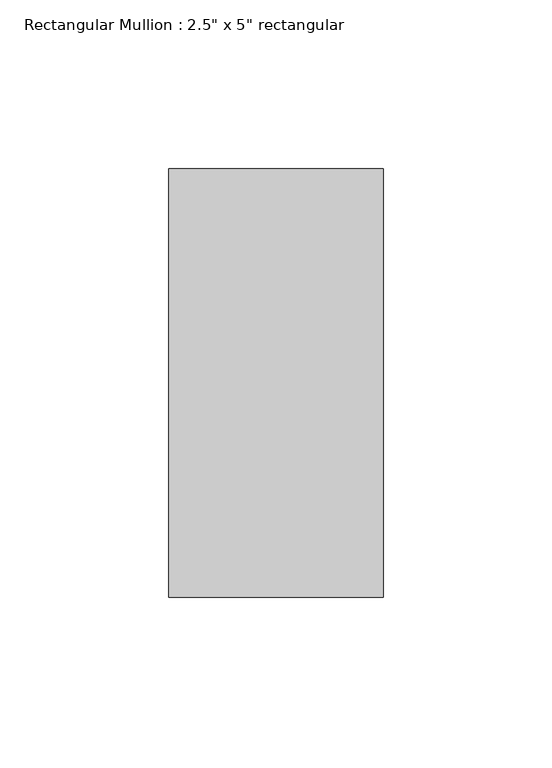
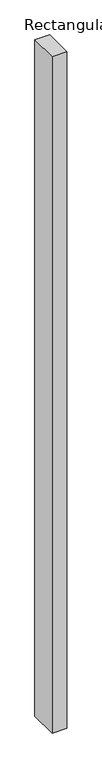
"""IFC4 building model written with IfcOpenShell, lengths in millimetres: member geometry."""

from ifc_helpers import new_model, si_unit, frame, origin, place, context, project, spatial, polyline, outline, extrude, source, transform, mapped, element, save


def member_3f395ae9(model_context):
    return source(origin(), model_context, "Body", "SweptSolid", [
        extrude(outline(polyline([(0.0, 63.5), (0.0, -63.5), (-63.5, -63.5), (-63.5, 63.5), (0.0, 63.5)])), frame((0.0, 0.0, -3048.0), z_axis=(0.0, 0.0, 1.0), x_axis=(1.0, 0.0, 0.0)), (0.0, 0.0, 1.0), 3048.0),
    ])


if __name__ == "__main__":
    model = new_model("IFC4")
    model_context = context("Model", 3, world=origin())
    ifc_project = project(units=[si_unit("LENGTHUNIT", "METRE", prefix="MILLI")], contexts=[model_context])
    site = spatial("IfcSite", under=ifc_project)
    building = spatial("IfcBuilding", under=site)
    placement = place(None, origin())
    member_shape = member_3f395ae9(model_context)
    element("IfcMember", 1, ObjectType="Rectangular Mullion : 2.5\" x 5\" rectangular", at=placement, inside=building, context=model_context, shape_type="MappedRepresentation", body=[
        mapped(member_shape, transform((0.0, 0.0, 0.0), x_axis=(1.0, 0.0, 0.0), y_axis=(0.0, 1.0, 0.0), z_axis=(0.0, 0.0, 1.0))),
    ])
    save(model, "model.ifc")

# Revit data of these elements
# Type "Rectangular Mullion : 2.5\" x 5\" rectangular"
#   built-in parameter 1007304 = 0.416667 (stored number, unit not read)
#   built-in parameter 1007301 = 0.104167 (stored number, unit not read)
#   built-in parameter 1007300 = 0.104167 (stored number, unit not read)
# Element 1 (IfcMember, "Rectangular Mullion : 2.5\" x 5\" rectangular")
#   Materials on its faces: "Iron, Ductile"
# Materials
#   "Iron, Ductile": class "Metal", colour RGB 0 0 0, transparency 0, Description = "Ductile cast iron", Cost = 0
